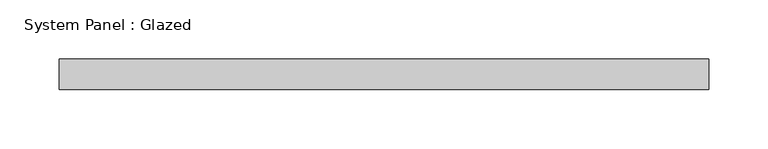
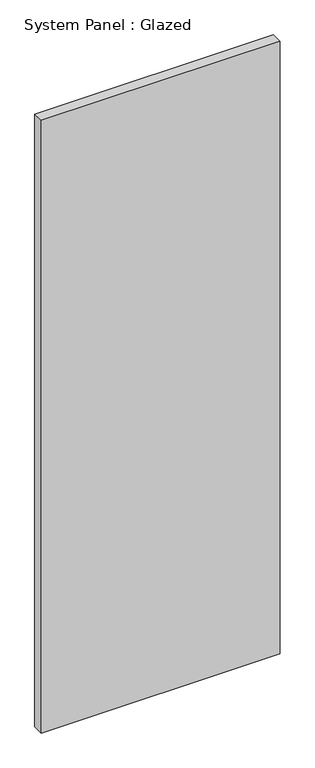
"""IFC4 building model written with IfcOpenShell, lengths in millimetres: plate geometry, System Panel : Glazed."""

from ifc_helpers import new_model, si_unit, origin, origin_with_axes, place, context, project, spatial, polyline, outline, extrude, source, transform, mapped, element, save


def system_panel_glazed_47776199(model_context):
    return source(origin(), model_context, "Body", "SweptSolid", [
        extrude(outline(polyline([(273.05, 19.05), (-273.05, 19.05), (-273.05, 44.45), (273.05, 44.45), (273.05, 19.05)])), origin_with_axes(), (0.0, 0.0, 1.0), 1480.0454815),
    ])


if __name__ == "__main__":
    model = new_model("IFC4")
    model_context = context("Model", 3, world=origin())
    ifc_project = project(units=[si_unit("LENGTHUNIT", "METRE", prefix="MILLI")], contexts=[model_context])
    site = spatial("IfcSite", under=ifc_project)
    building = spatial("IfcBuilding", under=site)
    placement = place(None, origin())
    system_panel_glazed_shape = system_panel_glazed_47776199(model_context)
    element("IfcPlate", 1, ObjectType="System Panel : Glazed", at=placement, inside=building, context=model_context, shape_type="MappedRepresentation", body=[
        mapped(system_panel_glazed_shape, transform((0.0, 0.0, 0.0), x_axis=(1.0, 0.0, 0.0), y_axis=(0.0, 1.0, 0.0), z_axis=(0.0, 0.0, 1.0))),
    ])
    save(model, "model.ifc")

# Revit data of these elements
# Type "System Panel : Glazed"
#   Construction Type Id = "GSP4R"
#   Analytic Construction = "1/8 in Pilkington single glazing"
#   Visual Light Transmittance = 0.9
#   Solar Heat Gain Coefficient = 0.86
#   Heat Transfer Coefficient (U) = 1.18115 BTU/(h·ft²·°F)
#   Define Thermal Properties by = 1
# Element 1 (IfcPlate, "System Panel : Glazed")
#   Materials on its faces: "Glass"
# Materials
#   "Glass": class "Glass", colour RGB 0 128 192, transparency 0.75, Description = "Soda Lime Glass", Cost = 0
